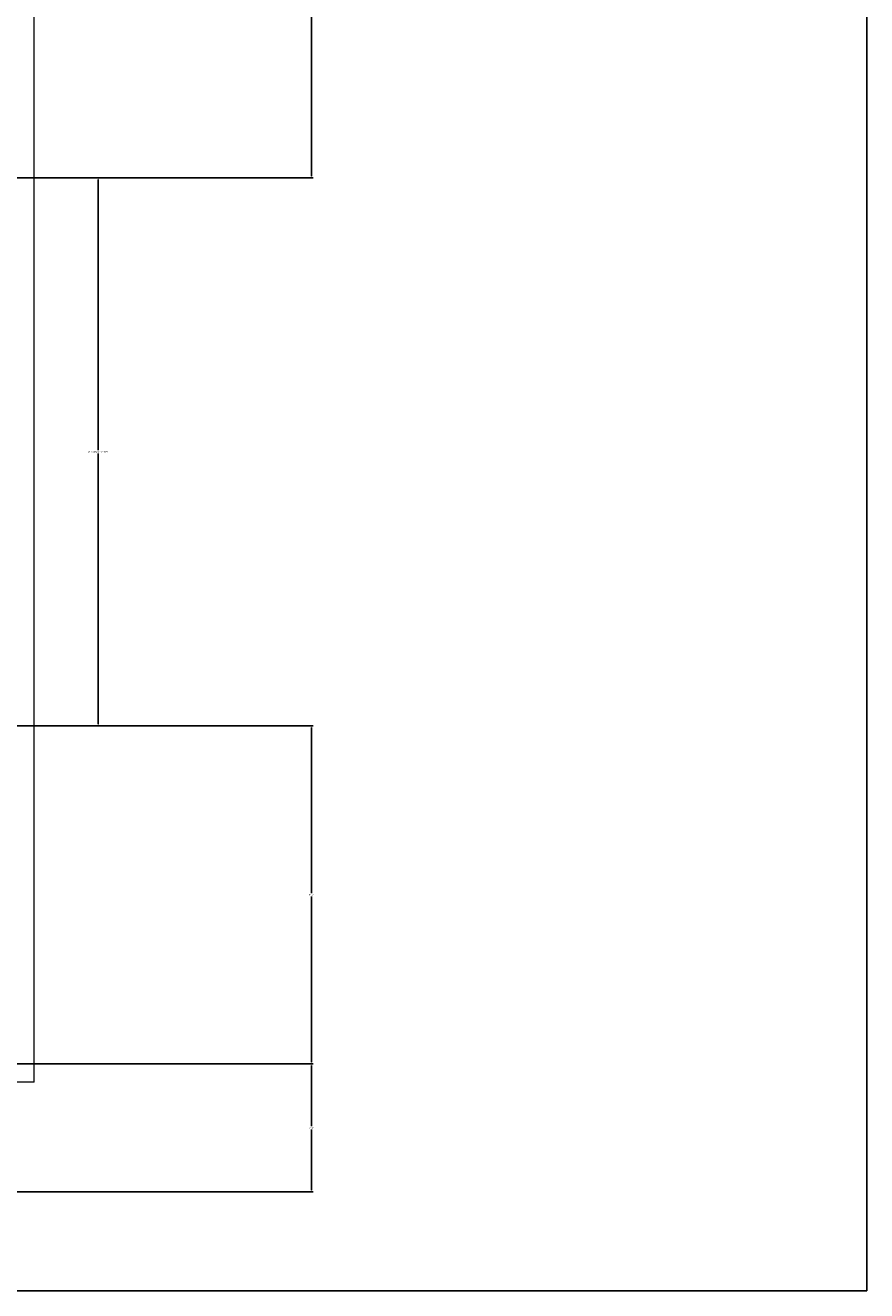
# Model space of a CAD drawing. Units: inches. Extents: x 311 to 815, y -527 to 136.
# Tile 13 of 21: x 723 to 815, y -507 to -368. Entities that reach past the tile are written whole.
import ezdxf

# ---------------------------------------------------------------- set-up
doc = ezdxf.new("R2010")
doc.units = ezdxf.units.IN
doc.header["$MEASUREMENT"] = 0
for name, color, linetype, lineweight in [('A-ANNO-DIMS', 1, 'Continuous', 18), ('A-ANNO-TTLB', 1, 'Continuous', 25), ('A-FLOR-EDGE', 1, 'Continuous', 18)]:
    doc.layers.add(name, color=color, linetype=linetype, lineweight=lineweight)
doc.styles.get("Standard").update_dxf_attribs({"font": 'arial.ttf'})
doc.dimstyles.get("Standard").update_dxf_attribs({"dimtxt": 0.18, "dimasz": 0.18, "dimexe": 0.18, "dimexo": 0.0625, "dimgap": 0.09, "dimtad": 0, "dimtih": 1, "dimtoh": 1, "dimdec": 1, "dimzin": 0, "dimdsep": 46, "dimlunit": 4, "dimtxsty": 'Standard', "dimcen": 0.09, "dimadec": 0, "dimazin": 0, "dimtfac": 1, "dimtdec": 1, "dimtofl": 0, "dimtmove": 0, "dimatfit": 3, "dimfxl": 1, "dimtolj": 1, "dimtzin": 0, "dimarcsym": 0})

# ---------------------------------------------------------------- blocks, each defined once
blk = doc.blocks.new('*D10')
at = {"layer": 'A-ANNO-DIMS', "color": 0, "lineweight": -2, "transparency": 16777216}
for p, q in [((722.39, -385.13), (731.5, -385.13)), ((731.32, -385.31), (731.32, -414.94)), ((731.32, -444.95), (731.32, -415.31)), ((722.39, -445.13), (731.5, -445.13))]:
    blk.add_line(p, q, dxfattribs=at)
at = {"layer": 'A-ANNO-DIMS', "color": 0, "transparency": 16777216}
for points in [[(731.29, -385.31), (731.35, -385.31), (731.32, -385.13)], [(731.29, -444.95), (731.35, -444.95), (731.32, -445.13)]]:
    blk.add_solid(points, dxfattribs=at)
at = {"layer": 'Defpoints', "color": 0, "transparency": 16777216}
for p in [(722.32, -385.13), (731.32, -385.13), (722.32, -445.13)]:
    blk.add_point(p, dxfattribs=at)
at = {"layer": 'A-ANNO-DIMS', "color": 0, "transparency": 16777216, "insert": (731.32, -415.13), "char_height": 0.18, "attachment_point": 5}
blk.add_mtext('\\A1;WINDOW 5\'-0" TYP.', dxfattribs=at)
blk = doc.blocks.new('*D24')
at = {"layer": 'A-ANNO-DIMS', "color": 0, "lineweight": -2, "transparency": 16777216}
for p, q in [((722.39, -482.13), (754.85, -482.13)), ((754.67, -482.31), (754.67, -488.95)), ((754.67, -495.95), (754.67, -489.31)), ((722.39, -496.13), (754.85, -496.13))]:
    blk.add_line(p, q, dxfattribs=at)
at = {"layer": 'A-ANNO-DIMS', "color": 0, "transparency": 16777216}
for points in [[(754.64, -482.31), (754.7, -482.31), (754.67, -482.13)], [(754.64, -495.95), (754.7, -495.95), (754.67, -496.13)]]:
    blk.add_solid(points, dxfattribs=at)
at = {"layer": 'Defpoints', "color": 0, "transparency": 16777216}
for p in [(722.32, -482.13), (722.33, -496.13), (754.67, -496.13)]:
    blk.add_point(p, dxfattribs=at)
at = {"layer": 'A-ANNO-DIMS', "color": 0, "transparency": 16777216, "insert": (754.67, -489.13), "char_height": 0.18, "attachment_point": 5}
blk.add_mtext('\\A1;1\'-2"', dxfattribs=at)
blk = doc.blocks.new('*D28')
at = {"layer": 'A-ANNO-DIMS', "color": 0, "lineweight": -2, "transparency": 16777216}
for p, q in [((722.39, -322.63), (754.85, -322.63)), ((754.67, -322.81), (754.67, -353.69)), ((754.67, -384.95), (754.67, -354.06)), ((722.39, -385.13), (754.85, -385.13))]:
    blk.add_line(p, q, dxfattribs=at)
at = {"layer": 'A-ANNO-DIMS', "color": 0, "transparency": 16777216}
for points in [[(754.64, -322.81), (754.7, -322.81), (754.67, -322.63)], [(754.64, -384.95), (754.7, -384.95), (754.67, -385.13)]]:
    blk.add_solid(points, dxfattribs=at)
at = {"layer": 'Defpoints', "color": 0, "transparency": 16777216}
for p in [(722.32, -322.63), (722.32, -385.13), (754.67, -385.13)]:
    blk.add_point(p, dxfattribs=at)
at = {"layer": 'A-ANNO-DIMS', "color": 0, "transparency": 16777216, "insert": (754.67, -353.88), "char_height": 0.18, "attachment_point": 5}
blk.add_mtext('\\A1;5\'-2 1/2"', dxfattribs=at)
blk = doc.blocks.new('*D30')
at = {"layer": 'A-ANNO-DIMS', "color": 0, "lineweight": -2, "transparency": 16777216}
for p, q in [((722.39, -445.13), (754.85, -445.13)), ((754.67, -445.31), (754.67, -463.45)), ((754.67, -481.95), (754.67, -463.81)), ((722.39, -482.13), (754.85, -482.13))]:
    blk.add_line(p, q, dxfattribs=at)
at = {"layer": 'A-ANNO-DIMS', "color": 0, "transparency": 16777216}
for points in [[(754.64, -445.31), (754.7, -445.31), (754.67, -445.13)], [(754.64, -481.95), (754.7, -481.95), (754.67, -482.13)]]:
    blk.add_solid(points, dxfattribs=at)
at = {"layer": 'Defpoints', "color": 0, "transparency": 16777216}
for p in [(722.32, -445.13), (754.67, -445.13), (722.32, -482.13)]:
    blk.add_point(p, dxfattribs=at)
at = {"layer": 'A-ANNO-DIMS', "color": 0, "transparency": 16777216, "insert": (754.67, -463.63), "char_height": 0.18, "attachment_point": 5}
blk.add_mtext('\\A1;3\'-1"', dxfattribs=at)

msp = doc.modelspace()

# ---------------------------------------------------------------- linework, layer by layer
at = {"layer": 'A-ANNO-TTLB'}
msp.add_lwpolyline([(310.67, 136.01), (815.43, 136.01), (815.43, -506.97), (310.67, -506.97)], close=True, dxfattribs=at)
at = {"layer": 'A-FLOR-EDGE'}
for q in [(724.32, 23.87), (408.32, -484.13)]:
    msp.add_line((724.32, -484.13), q, dxfattribs=at)

# ---------------------------------------------------------------- dimensions: what is measured, and where the dimension line sits
at = {"layer": 'A-ANNO-DIMS'}
for base, p1, p2, picture, middle in [((754.67, -385.13), (722.32, -322.63), (722.32, -385.13), '*D28', (754.67, -353.88)), ((754.67, -445.13), (722.32, -482.13), (722.32, -445.13), '*D30', (754.67, -463.63)), ((754.67, -496.13), (722.32, -482.13), (722.33, -496.13), '*D24', (754.67, -489.13))]:
    dim = msp.add_linear_dim(base=base, p1=p1, p2=p2, angle=90, dimstyle='Standard', override={"dimdec": 1, "dimlfac": 1, "dimrnd": 0, "dimzin": 1, "dimdsep": 46, "dimlunit": 4, "dimfrac": 2}, dxfattribs=at)
    dim.commit()
    dim.dimension.update_dxf_attribs({"geometry": picture, "text_midpoint": middle})
dim = msp.add_linear_dim(base=(731.32, -385.13), p1=(722.32, -445.13), p2=(722.32, -385.13), angle=90, text='WINDOW <> TYP.', dimstyle='Standard', override={"dimdec": 1, "dimlfac": 1, "dimrnd": 0, "dimzin": 1, "dimdsep": 46, "dimlunit": 4, "dimfrac": 2}, dxfattribs=at)
dim.commit()
dim.dimension.update_dxf_attribs({"geometry": '*D10', "text_midpoint": (731.32, -415.13)})

doc.saveas('drawing.dxf')
